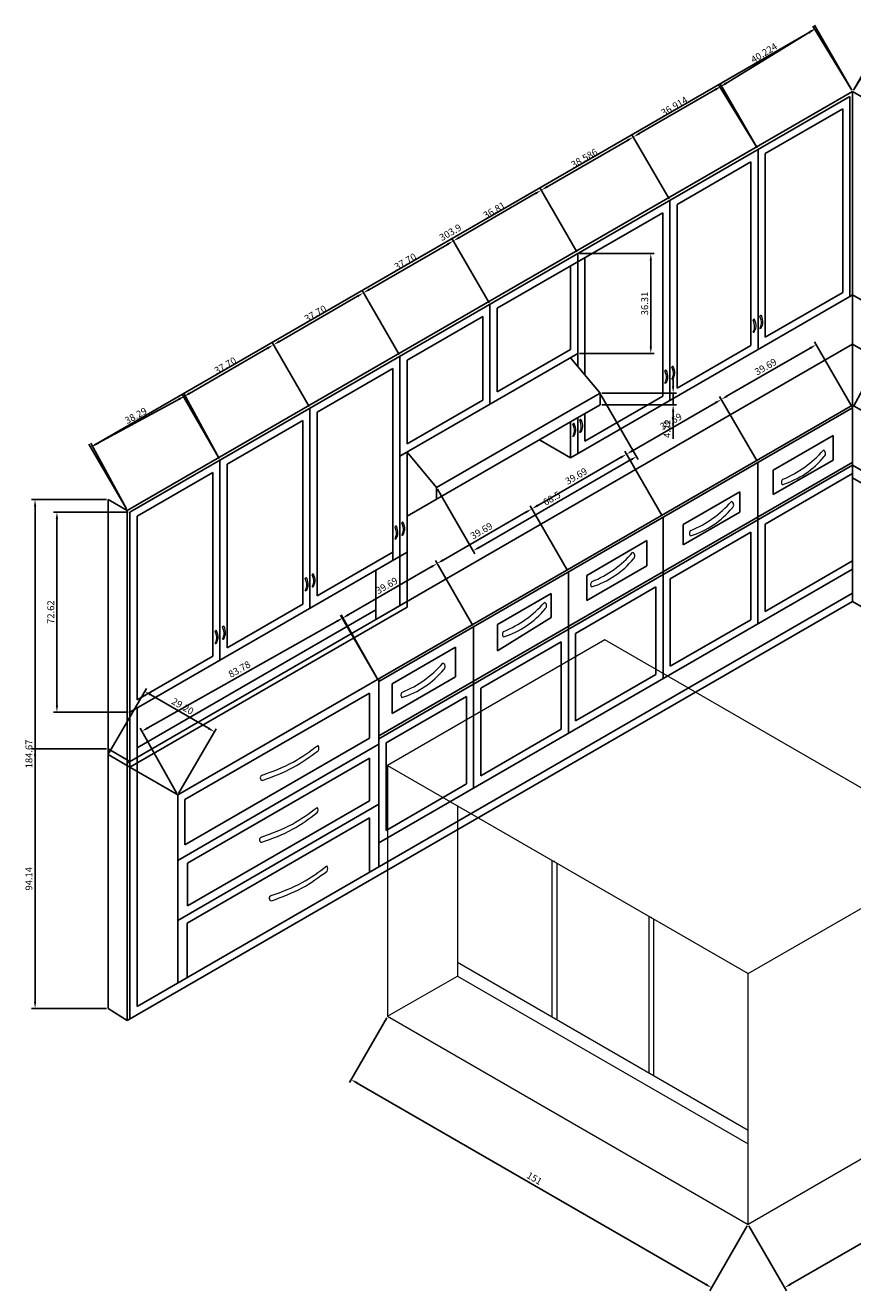
# Model space of a CAD drawing. Units: centimetres. Extents: x 21667 to 22807, y 15845 to 16565.
# Tile 3 of 4: x 22275 to 22575, y 16106 to 16565. Entities that reach past the tile are written whole.
import ezdxf

# ---------------------------------------------------------------- set-up
doc = ezdxf.new("R2010")
doc.units = ezdxf.units.CM
for name, color, linetype, lineweight in [('A-ANNO-DIMS', 2, 'Continuous', 18), ('A-ANNO-NPLT', 8, 'Continuous', 13), ('A-FURN', 8, 'Continuous', 18), ('A-FURN-CASE', 7, 'Continuous', 25), ('A-FURN-HDWR', 8, 'Continuous', 13)]:
    doc.layers.add(name, color=color, linetype=linetype, lineweight=lineweight)
doc.styles.get("Standard").update_dxf_attribs({"font": 'arial.ttf'})
doc.dimstyles.new('ISO-25', dxfattribs={"dimtxt": 2.5, "dimasz": 2.5, "dimexe": 1.25, "dimexo": 0.625, "dimtad": 1, "dimtxsty": 'Standard', "dimcen": 2.5, "dimadec": 0, "dimazin": 0, "dimtfac": 1, "dimtmove": 0, "dimatfit": 3, "dimfxl": 1, "dimarcsym": 0})

# ---------------------------------------------------------------- blocks, each defined once
blk = doc.blocks.new('hanger')
for centre, radius, start, end in [((22344.01, 16340.62), 0.329, 55.972, 165.7251), ((22343.56, 16337.35), 1.11, 276.778, 304.9191)]:
    blk.add_arc(centre, radius, start, end)
for points, knots in [([(22343.69, 16336.25), (22343.94, 16336.83), (22344.57, 16338.28), (22344.02, 16339.79), (22343.69, 16340.7)], [0, 0, 0, 0, 1.834135, 4.5977, 4.5977, 4.5977, 4.5977]), ([(22344.2, 16336.44), (22344.45, 16337.04), (22345.07, 16338.5), (22344.52, 16340.01), (22344.2, 16340.89)], [0, 0, 0, 0, 1.89598, 4.599425, 4.599425, 4.599425, 4.599425])]:
    blk.add_open_spline(points, degree=3, knots=knots)
blk = doc.blocks.new('tabl e3')
for p, q in [((22512.57, 16212.95), (22433.76, 16167.45)), ((22643.34, 16137.45), (22512.57, 16212.95)), ((22433.76, 16167.45), (22564.53, 16091.95)), ((22433.76, 16167.45), (22433.76, 16076.45)), ((22459.07, 16152.84), (22459.07, 16091.06)), ((22564.53, 16091.95), (22643.34, 16137.45)), ((22643.34, 16137.45), (22643.34, 16046.45)), ((22493.36, 16133.04), (22493.36, 16076.26)), ((22495.09, 16132.04), (22495.09, 16075.26)), ((22528.51, 16112.74), (22528.51, 16055.97)), ((22530.25, 16111.74), (22530.25, 16054.97)), ((22459.07, 16096.06), (22564.53, 16035.17)), ((22433.76, 16076.45), (22459.07, 16091.06)), ((22459.07, 16091.06), (22564.53, 16030.17)), ((22564.53, 16000.95), (22564.53, 16091.95)), ((22433.76, 16076.45), (22564.53, 16000.95)), ((22643.34, 16046.45), (22564.53, 16000.95))]:
    blk.add_line(p, q)
for p in [(22494.23, 16132.54), (22529.38, 16112.24)]:
    blk.add_point(p)
blk = doc.blocks.new('PULL-KNOB-D')
for centre, radius, start, end in [((19.64, 11.69), 1.63, 325.6763, 37.1687), ((0.97, 0.96), 0.968, 101.3534, 261.4916)]:
    blk.add_arc(centre, radius, start, end)
for points in [[(0.78, 1.91), (4.6, 3.31), (11.83, 5.95), (18.02, 10.52), (20.94, 12.67)], [(0.82, 0), (4.64, 1.4), (11.87, 4.05), (18.07, 8.61), (20.99, 10.77)]]:
    blk.add_open_spline(points, degree=3, knots=[0, 0, 0, 0, 12.131271, 22.961741, 22.961741, 22.961741, 22.961741])
blk = doc.blocks.new('DRAWER-PULL')
for centre, radius, start, end in [((-9.25, 30.72), 32.2, 287.3997, 320.4809), ((-14.25, 38.11), 39.06, 292.2568, 319.0454), ((14.72, 11.27), 1.35, 309.9814, 67.0584), ((1.29, 0.92), 1.29, 125.3328, 225.1316)]:
    blk.add_arc(centre, radius, start, end)
blk = doc.blocks.new('*D26')
at = {"layer": 'A-ANNO-DIMS', "color": 0, "lineweight": -2, "transparency": 16777216}
for p, q in [((22574.64, 16541.62), (22561.08, 16565.11)), ((22300.7, 16413.33), (22559.54, 16562.77)), ((22311.47, 16389.67), (22297.91, 16413.17))]:
    blk.add_line(p, q, dxfattribs=at)
at = {"layer": 'A-ANNO-DIMS', "color": 0, "transparency": 16777216}
for points in [[(22559.33, 16563.14), (22559.75, 16562.41), (22561.7, 16564.02)], [(22300.49, 16413.69), (22300.9, 16412.97), (22298.53, 16412.08)]]:
    blk.add_solid(points, dxfattribs=at)
at = {"layer": 'Defpoints', "color": 0, "transparency": 16777216}
for p in [(22561.7, 16564.02), (22574.95, 16541.07), (22311.78, 16389.13)]:
    blk.add_point(p, dxfattribs=at)
at = {"layer": 'A-ANNO-DIMS', "color": 0, "transparency": 16777216, "insert": (22429.17, 16489.7), "char_height": 2.5, "attachment_point": 5, "rotation": 30}
blk.add_mtext('303.9', dxfattribs=at)
blk = doc.blocks.new('*D27')
at = {"layer": 'A-ANNO-DIMS', "color": 0, "lineweight": -2, "transparency": 16777216}
for p, q in [((22575.26, 16541.62), (22588.83, 16565.11)), ((22590.37, 16562.77), (22793.02, 16445.77)), ((22782.24, 16422.12), (22795.81, 16445.61))]:
    blk.add_line(p, q, dxfattribs=at)
at = {"layer": 'A-ANNO-DIMS', "color": 0, "transparency": 16777216}
for points in [[(22590.58, 16563.14), (22590.16, 16562.41), (22588.2, 16564.02)], [(22793.23, 16446.14), (22792.81, 16445.41), (22795.18, 16444.52)]]:
    blk.add_solid(points, dxfattribs=at)
at = {"layer": 'Defpoints', "color": 0, "transparency": 16777216}
for p in [(22574.95, 16541.07), (22795.18, 16444.52), (22781.93, 16421.57)]:
    blk.add_point(p, dxfattribs=at)
at = {"layer": 'A-ANNO-DIMS', "color": 0, "transparency": 16777216, "insert": (22692.64, 16505.92), "char_height": 2.5, "attachment_point": 5, "rotation": 330}
blk.add_mtext('239', dxfattribs=at)
blk = doc.blocks.new('*D28')
at = {"layer": 'A-ANNO-DIMS', "color": 0, "lineweight": -2, "transparency": 16777216}
for p, q in [((22304.23, 16393.13), (22277.1, 16393.13)), ((22278.35, 16210.96), (22278.35, 16390.63)), ((22304.23, 16208.46), (22277.1, 16208.46))]:
    blk.add_line(p, q, dxfattribs=at)
at = {"layer": 'A-ANNO-DIMS', "color": 0, "transparency": 16777216}
for points in [[(22277.94, 16390.63), (22278.77, 16390.63), (22278.35, 16393.13)], [(22277.94, 16210.96), (22278.77, 16210.96), (22278.35, 16208.46)]]:
    blk.add_solid(points, dxfattribs=at)
at = {"layer": 'Defpoints', "color": 0, "transparency": 16777216}
for p in [(22278.35, 16393.13), (22304.85, 16393.13), (22304.85, 16208.46)]:
    blk.add_point(p, dxfattribs=at)
at = {"layer": 'A-ANNO-DIMS', "color": 0, "transparency": 16777216, "insert": (22276.45, 16300.8), "char_height": 2.5, "attachment_point": 5, "rotation": 90}
blk.add_mtext('184.67', dxfattribs=at)
blk = doc.blocks.new('*D29')
at = {"layer": 'A-ANNO-DIMS', "color": 0, "lineweight": -2, "transparency": 16777216}
for p, q in [((22304.23, 16302.61), (22277.1, 16302.61)), ((22278.35, 16210.96), (22278.35, 16300.11)), ((22304.23, 16208.46), (22277.1, 16208.46))]:
    blk.add_line(p, q, dxfattribs=at)
at = {"layer": 'A-ANNO-DIMS', "color": 0, "transparency": 16777216}
for points in [[(22277.94, 16300.11), (22278.77, 16300.11), (22278.35, 16302.61)], [(22277.94, 16210.96), (22278.77, 16210.96), (22278.35, 16208.46)]]:
    blk.add_solid(points, dxfattribs=at)
at = {"layer": 'Defpoints', "color": 0, "transparency": 16777216}
for p in [(22278.35, 16302.61), (22304.85, 16302.61), (22304.85, 16208.46)]:
    blk.add_point(p, dxfattribs=at)
at = {"layer": 'A-ANNO-DIMS', "color": 0, "transparency": 16777216, "insert": (22276.45, 16255.53), "char_height": 2.5, "attachment_point": 5, "rotation": 90}
blk.add_mtext('94.14', dxfattribs=at)
blk = doc.blocks.new('*D30')
at = {"layer": 'A-ANNO-DIMS', "color": 0, "lineweight": -2, "transparency": 16777216}
for p, q in [((22312.16, 16388.56), (22285.03, 16388.56)), ((22286.28, 16318.44), (22286.28, 16386.06)), ((22312.16, 16315.94), (22285.03, 16315.94))]:
    blk.add_line(p, q, dxfattribs=at)
at = {"layer": 'A-ANNO-DIMS', "color": 0, "transparency": 16777216}
for points in [[(22285.86, 16386.06), (22286.7, 16386.06), (22286.28, 16388.56)], [(22285.86, 16318.44), (22286.7, 16318.44), (22286.28, 16315.94)]]:
    blk.add_solid(points, dxfattribs=at)
at = {"layer": 'Defpoints', "color": 0, "transparency": 16777216}
for p in [(22286.28, 16388.56), (22312.78, 16388.56), (22312.78, 16315.94)]:
    blk.add_point(p, dxfattribs=at)
at = {"layer": 'A-ANNO-DIMS', "color": 0, "transparency": 16777216, "insert": (22284.38, 16352.25), "char_height": 2.5, "attachment_point": 5, "rotation": 90}
blk.add_mtext('72.62', dxfattribs=at)
blk = doc.blocks.new('*D31')
at = {"layer": 'A-ANNO-DIMS', "color": 0, "lineweight": -2, "transparency": 16777216}
for p, q in [((22483.65, 16431.12), (22497.21, 16407.63)), ((22494.42, 16407.46), (22439.42, 16375.71)), ((22424.32, 16396.87), (22437.88, 16373.38))]:
    blk.add_line(p, q, dxfattribs=at)
at = {"layer": 'A-ANNO-DIMS', "color": 0, "transparency": 16777216}
for points in [[(22494.21, 16407.82), (22494.63, 16407.1), (22496.58, 16408.71)], [(22439.21, 16376.07), (22439.63, 16375.35), (22437.26, 16374.46)]]:
    blk.add_solid(points, dxfattribs=at)
at = {"layer": 'Defpoints', "color": 0, "transparency": 16777216}
for p in [(22483.33, 16431.66), (22424.01, 16397.41), (22437.26, 16374.46)]:
    blk.add_point(p, dxfattribs=at)
at = {"layer": 'A-ANNO-DIMS', "color": 0, "transparency": 16777216, "insert": (22465.97, 16393.23), "char_height": 2.5, "attachment_point": 5, "rotation": 30}
blk.add_mtext('68.5', dxfattribs=at)
blk = doc.blocks.new('*D34')
at = {"layer": 'A-ANNO-DIMS', "color": 0, "lineweight": -2, "transparency": 16777216}
for p, q in [((22405.95, 16205.11), (22392.39, 16181.62)), ((22521.62, 16108.45), (22395.18, 16181.45)), ((22536.72, 16129.61), (22523.16, 16106.12))]:
    blk.add_line(p, q, dxfattribs=at)
at = {"layer": 'A-ANNO-DIMS', "color": 0, "transparency": 16777216}
for points in [[(22395.39, 16181.81), (22394.97, 16181.09), (22393.01, 16182.7)], [(22521.83, 16108.81), (22521.41, 16108.09), (22523.78, 16107.2)]]:
    blk.add_solid(points, dxfattribs=at)
at = {"layer": 'Defpoints', "color": 0, "transparency": 16777216}
for p in [(22406.26, 16205.65), (22393.01, 16182.7), (22537.03, 16130.15)]:
    blk.add_point(p, dxfattribs=at)
at = {"layer": 'A-ANNO-DIMS', "color": 0, "transparency": 16777216, "insert": (22459.35, 16146.59), "char_height": 2.5, "attachment_point": 5, "rotation": 330}
blk.add_mtext('151', dxfattribs=at)
blk = doc.blocks.new('*D35')
at = {"layer": 'A-ANNO-DIMS', "color": 0, "lineweight": -2, "transparency": 16777216}
for p, q in [((22616.15, 16175.11), (22629.72, 16151.62)), ((22626.93, 16151.45), (22552.45, 16108.45)), ((22537.35, 16129.61), (22550.91, 16106.12))]:
    blk.add_line(p, q, dxfattribs=at)
at = {"layer": 'A-ANNO-DIMS', "color": 0, "transparency": 16777216}
for points in [[(22626.72, 16151.81), (22627.14, 16151.09), (22629.09, 16152.7)], [(22552.24, 16108.81), (22552.66, 16108.09), (22550.28, 16107.2)]]:
    blk.add_solid(points, dxfattribs=at)
at = {"layer": 'Defpoints', "color": 0, "transparency": 16777216}
for p in [(22615.84, 16175.65), (22537.03, 16130.15), (22550.28, 16107.2)]:
    blk.add_point(p, dxfattribs=at)
at = {"layer": 'A-ANNO-DIMS', "color": 0, "transparency": 16777216, "insert": (22588.74, 16131.59), "char_height": 2.5, "attachment_point": 5, "rotation": 30}
blk.add_mtext('91', dxfattribs=at)
blk = doc.blocks.new('*D54')
at = {"layer": 'A-ANNO-DIMS', "color": 0, "lineweight": -2, "transparency": 16777216}
for p, q in [((22301.33, 16413.61), (22330.58, 16429.5)), ((22345.13, 16407.95), (22332.18, 16431.79)), ((22311.48, 16389.68), (22298.54, 16413.52))]:
    blk.add_line(p, q, dxfattribs=at)
at = {"layer": 'A-ANNO-DIMS', "color": 0, "transparency": 16777216}
for points in [[(22330.38, 16429.86), (22330.78, 16429.13), (22332.78, 16430.69)], [(22301.13, 16413.98), (22301.53, 16413.25), (22299.13, 16412.42)]]:
    blk.add_solid(points, dxfattribs=at)
at = {"layer": 'Defpoints', "color": 0, "transparency": 16777216}
for p in [(22332.78, 16430.69), (22345.43, 16407.4), (22311.78, 16389.13)]:
    blk.add_point(p, dxfattribs=at)
at = {"layer": 'A-ANNO-DIMS', "color": 0, "transparency": 16777216, "insert": (22315.05, 16423.23), "char_height": 2.5, "attachment_point": 5, "rotation": 28.5034}
blk.add_mtext('38.29', dxfattribs=at)
blk = doc.blocks.new('*D55')
at = {"layer": 'A-ANNO-DIMS', "color": 0, "lineweight": -2, "transparency": 16777216}
for p, q in [((22377.76, 16426.79), (22364.2, 16450.28)), ((22334.34, 16431.6), (22362.66, 16447.95)), ((22345.11, 16407.95), (22331.55, 16431.44))]:
    blk.add_line(p, q, dxfattribs=at)
at = {"layer": 'A-ANNO-DIMS', "color": 0, "transparency": 16777216}
for points in [[(22362.45, 16448.31), (22362.87, 16447.59), (22364.82, 16449.2)], [(22334.13, 16431.96), (22334.55, 16431.24), (22332.18, 16430.35)]]:
    blk.add_solid(points, dxfattribs=at)
at = {"layer": 'Defpoints', "color": 0, "transparency": 16777216}
for p in [(22364.82, 16449.2), (22378.07, 16426.25), (22345.43, 16407.4)]:
    blk.add_point(p, dxfattribs=at)
at = {"layer": 'A-ANNO-DIMS', "color": 0, "transparency": 16777216, "insert": (22347.55, 16441.43), "char_height": 2.5, "attachment_point": 5, "rotation": 30}
blk.add_mtext('37.70', dxfattribs=at)
blk = doc.blocks.new('*D56')
at = {"layer": 'A-ANNO-DIMS', "color": 0, "lineweight": -2, "transparency": 16777216}
for p, q in [((22410.41, 16445.64), (22396.84, 16469.13)), ((22366.99, 16450.45), (22395.3, 16466.8)), ((22377.76, 16426.79), (22364.2, 16450.28))]:
    blk.add_line(p, q, dxfattribs=at)
at = {"layer": 'A-ANNO-DIMS', "color": 0, "transparency": 16777216}
for points in [[(22395.1, 16467.16), (22395.51, 16466.44), (22397.47, 16468.05)], [(22366.78, 16450.81), (22367.2, 16450.09), (22364.82, 16449.2)]]:
    blk.add_solid(points, dxfattribs=at)
at = {"layer": 'Defpoints', "color": 0, "transparency": 16777216}
for p in [(22397.47, 16468.05), (22410.72, 16445.1), (22378.07, 16426.25)]:
    blk.add_point(p, dxfattribs=at)
at = {"layer": 'A-ANNO-DIMS', "color": 0, "transparency": 16777216, "insert": (22380.2, 16460.27), "char_height": 2.5, "attachment_point": 5, "rotation": 30}
blk.add_mtext('37.70', dxfattribs=at)
blk = doc.blocks.new('*D57')
at = {"layer": 'A-ANNO-DIMS', "color": 0, "lineweight": -2, "transparency": 16777216}
for p, q in [((22443.05, 16464.49), (22429.49, 16487.98)), ((22399.63, 16469.3), (22427.95, 16485.65)), ((22410.41, 16445.64), (22396.84, 16469.13))]:
    blk.add_line(p, q, dxfattribs=at)
at = {"layer": 'A-ANNO-DIMS', "color": 0, "transparency": 16777216}
for points in [[(22427.74, 16486.01), (22428.16, 16485.29), (22430.12, 16486.9)], [(22399.43, 16469.66), (22399.84, 16468.94), (22397.47, 16468.05)]]:
    blk.add_solid(points, dxfattribs=at)
at = {"layer": 'Defpoints', "color": 0, "transparency": 16777216}
for p in [(22430.12, 16486.9), (22443.37, 16463.95), (22410.72, 16445.1)]:
    blk.add_point(p, dxfattribs=at)
at = {"layer": 'A-ANNO-DIMS', "color": 0, "transparency": 16777216, "insert": (22412.84, 16479.12), "char_height": 2.5, "attachment_point": 5, "rotation": 30}
blk.add_mtext('37.70', dxfattribs=at)
blk = doc.blocks.new('*D58')
at = {"layer": 'A-ANNO-DIMS', "color": 0, "lineweight": -2, "transparency": 16777216}
for p, q in [((22474.93, 16482.89), (22461.37, 16506.39)), ((22432.28, 16488.15), (22459.83, 16504.05)), ((22443.05, 16464.49), (22429.49, 16487.98))]:
    blk.add_line(p, q, dxfattribs=at)
at = {"layer": 'A-ANNO-DIMS', "color": 0, "transparency": 16777216}
for points in [[(22459.62, 16504.41), (22460.04, 16503.69), (22461.99, 16505.3)], [(22432.07, 16488.51), (22432.49, 16487.79), (22430.12, 16486.9)]]:
    blk.add_solid(points, dxfattribs=at)
at = {"layer": 'Defpoints', "color": 0, "transparency": 16777216}
for p in [(22461.99, 16505.3), (22475.24, 16482.35), (22443.37, 16463.95)]:
    blk.add_point(p, dxfattribs=at)
at = {"layer": 'A-ANNO-DIMS', "color": 0, "transparency": 16777216, "insert": (22445.1, 16497.75), "char_height": 2.5, "attachment_point": 5, "rotation": 30}
blk.add_mtext('36.81', dxfattribs=at)
blk = doc.blocks.new('*D59')
at = {"layer": 'A-ANNO-DIMS', "color": 0, "lineweight": -2, "transparency": 16777216}
for p, q in [((22508.35, 16502.19), (22494.78, 16525.68)), ((22464.16, 16506.55), (22493.24, 16523.35)), ((22474.93, 16482.89), (22461.37, 16506.39))]:
    blk.add_line(p, q, dxfattribs=at)
at = {"layer": 'A-ANNO-DIMS', "color": 0, "transparency": 16777216}
for points in [[(22493.04, 16523.71), (22493.45, 16522.98), (22495.41, 16524.6)], [(22463.95, 16506.91), (22464.37, 16506.19), (22461.99, 16505.3)]]:
    blk.add_solid(points, dxfattribs=at)
at = {"layer": 'Defpoints', "color": 0, "transparency": 16777216}
for p in [(22495.41, 16524.6), (22508.66, 16501.65), (22475.24, 16482.35)]:
    blk.add_point(p, dxfattribs=at)
at = {"layer": 'A-ANNO-DIMS', "color": 0, "transparency": 16777216, "insert": (22477.75, 16516.6), "char_height": 2.5, "attachment_point": 5, "rotation": 30}
blk.add_mtext('38.586', dxfattribs=at)
blk = doc.blocks.new('*D60')
at = {"layer": 'A-ANNO-DIMS', "color": 0, "lineweight": -2, "transparency": 16777216}
for p, q in [((22540.32, 16520.64), (22526.75, 16544.14)), ((22497.57, 16525.85), (22525.21, 16541.8)), ((22508.35, 16502.19), (22494.78, 16525.68))]:
    blk.add_line(p, q, dxfattribs=at)
at = {"layer": 'A-ANNO-DIMS', "color": 0, "transparency": 16777216}
for points in [[(22525, 16542.16), (22525.42, 16541.44), (22527.38, 16543.05)], [(22497.37, 16526.21), (22497.78, 16525.48), (22495.41, 16524.6)]]:
    blk.add_solid(points, dxfattribs=at)
at = {"layer": 'Defpoints', "color": 0, "transparency": 16777216}
for p in [(22527.38, 16543.05), (22540.63, 16520.1), (22508.66, 16501.65)]:
    blk.add_point(p, dxfattribs=at)
at = {"layer": 'A-ANNO-DIMS', "color": 0, "transparency": 16777216, "insert": (22510.44, 16535.47), "char_height": 2.5, "attachment_point": 5, "rotation": 30}
blk.add_mtext('36.914', dxfattribs=at)
blk = doc.blocks.new('*D61')
at = {"layer": 'A-ANNO-DIMS', "color": 0, "lineweight": -2, "transparency": 16777216}
for p, q in [((22528.94, 16544.02), (22559, 16562.38)), ((22574.63, 16541.61), (22560.48, 16564.75)), ((22540.3, 16520.64), (22526.16, 16543.78))]:
    blk.add_line(p, q, dxfattribs=at)
at = {"layer": 'A-ANNO-DIMS', "color": 0, "transparency": 16777216}
for points in [[(22558.78, 16562.74), (22559.22, 16562.03), (22561.14, 16563.69)], [(22528.73, 16544.38), (22529.16, 16543.66), (22526.81, 16542.72)]]:
    blk.add_solid(points, dxfattribs=at)
at = {"layer": 'Defpoints', "color": 0, "transparency": 16777216}
for p in [(22561.14, 16563.69), (22574.95, 16541.07), (22540.63, 16520.1)]:
    blk.add_point(p, dxfattribs=at)
at = {"layer": 'A-ANNO-DIMS', "color": 0, "transparency": 16777216, "insert": (22542.98, 16554.82), "char_height": 2.5, "attachment_point": 5, "rotation": 31.4246}
blk.add_mtext('40.224', dxfattribs=at)
blk = doc.blocks.new('*D62')
at = {"layer": 'A-ANNO-DIMS', "color": 0, "lineweight": -2, "transparency": 16777216}
for p, q in [((22575.28, 16541.61), (22589.49, 16564.71)), ((22590.96, 16562.34), (22613.38, 16548.56)), ((22601.95, 16525.21), (22616.16, 16548.31))]:
    blk.add_line(p, q, dxfattribs=at)
at = {"layer": 'A-ANNO-DIMS', "color": 0, "transparency": 16777216}
for points in [[(22591.18, 16562.69), (22590.74, 16561.99), (22588.83, 16563.65)], [(22613.59, 16548.91), (22613.16, 16548.2), (22615.51, 16547.25)]]:
    blk.add_solid(points, dxfattribs=at)
at = {"layer": 'Defpoints', "color": 0, "transparency": 16777216}
for p in [(22615.51, 16547.25), (22574.95, 16541.07), (22601.63, 16524.67)]:
    blk.add_point(p, dxfattribs=at)
at = {"layer": 'A-ANNO-DIMS', "color": 0, "transparency": 16777216, "insert": (22603.16, 16557.07), "char_height": 2.5, "attachment_point": 5, "rotation": 328.4151}
blk.add_mtext('31.31', dxfattribs=at)
blk = doc.blocks.new('*D69')
at = {"layer": 'A-ANNO-DIMS', "color": 0, "lineweight": -2, "transparency": 16777216}
for p, q in [((22402.78, 16327.62), (22389.46, 16351.25)), ((22319.27, 16310.25), (22387.9, 16348.93)), ((22329.79, 16286.48), (22316.48, 16310.11))]:
    blk.add_line(p, q, dxfattribs=at)
at = {"layer": 'A-ANNO-DIMS', "color": 0, "transparency": 16777216}
for points in [[(22387.69, 16349.3), (22388.1, 16348.57), (22390.08, 16350.16)], [(22319.06, 16310.61), (22319.47, 16309.89), (22317.09, 16309.02)]]:
    blk.add_solid(points, dxfattribs=at)
at = {"layer": 'Defpoints', "color": 0, "transparency": 16777216}
for p in [(22390.08, 16350.16), (22403.09, 16327.08), (22330.1, 16285.94)]:
    blk.add_point(p, dxfattribs=at)
at = {"layer": 'A-ANNO-DIMS', "color": 0, "transparency": 16777216, "insert": (22352.65, 16331.25), "char_height": 2.5, "attachment_point": 5, "rotation": 29.4078}
blk.add_mtext('83.78', dxfattribs=at)
blk = doc.blocks.new('*D70')
at = {"layer": 'A-ANNO-DIMS', "color": 0, "lineweight": -2, "transparency": 16777216}
for p, q in [((22392, 16351.28), (22422.05, 16368.62)), ((22437.15, 16347.46), (22423.59, 16370.95)), ((22402.78, 16327.62), (22389.21, 16351.11))]:
    blk.add_line(p, q, dxfattribs=at)
at = {"layer": 'A-ANNO-DIMS', "color": 0, "transparency": 16777216}
for points in [[(22421.84, 16368.98), (22422.25, 16368.26), (22424.21, 16369.87)], [(22391.8, 16351.64), (22392.21, 16350.92), (22389.84, 16350.03)]]:
    blk.add_solid(points, dxfattribs=at)
at = {"layer": 'Defpoints', "color": 0, "transparency": 16777216}
for p in [(22424.21, 16369.87), (22437.46, 16346.92), (22403.09, 16327.08)]:
    blk.add_point(p, dxfattribs=at)
at = {"layer": 'A-ANNO-DIMS', "color": 0, "transparency": 16777216, "insert": (22406.07, 16361.6), "char_height": 2.5, "attachment_point": 5, "rotation": 30}
blk.add_mtext('39.69', dxfattribs=at)
blk = doc.blocks.new('*D71')
at = {"layer": 'A-ANNO-DIMS', "color": 0, "lineweight": -2, "transparency": 16777216}
for p, q in [((22471.52, 16367.31), (22457.96, 16390.8)), ((22426.38, 16371.12), (22456.42, 16388.47)), ((22437.15, 16347.46), (22423.59, 16370.95))]:
    blk.add_line(p, q, dxfattribs=at)
at = {"layer": 'A-ANNO-DIMS', "color": 0, "transparency": 16777216}
for points in [[(22456.21, 16388.83), (22456.63, 16388.11), (22458.58, 16389.72)], [(22426.17, 16371.48), (22426.58, 16370.76), (22424.21, 16369.87)]]:
    blk.add_solid(points, dxfattribs=at)
at = {"layer": 'Defpoints', "color": 0, "transparency": 16777216}
for p in [(22458.58, 16389.72), (22471.83, 16366.77), (22437.46, 16346.92)]:
    blk.add_point(p, dxfattribs=at)
at = {"layer": 'A-ANNO-DIMS', "color": 0, "transparency": 16777216, "insert": (22440.45, 16381.44), "char_height": 2.5, "attachment_point": 5, "rotation": 30}
blk.add_mtext('39.69', dxfattribs=at)
blk = doc.blocks.new('*D72')
at = {"layer": 'A-ANNO-DIMS', "color": 0, "lineweight": -2, "transparency": 16777216}
for p, q in [((22505.89, 16387.15), (22492.33, 16410.64)), ((22460.75, 16390.97), (22490.79, 16408.31)), ((22471.52, 16367.31), (22457.96, 16390.8))]:
    blk.add_line(p, q, dxfattribs=at)
at = {"layer": 'A-ANNO-DIMS', "color": 0, "transparency": 16777216}
for points in [[(22490.58, 16408.67), (22491, 16407.95), (22492.96, 16409.56)], [(22460.54, 16391.33), (22460.96, 16390.61), (22458.58, 16389.72)]]:
    blk.add_solid(points, dxfattribs=at)
at = {"layer": 'Defpoints', "color": 0, "transparency": 16777216}
for p in [(22492.96, 16409.56), (22506.21, 16386.61), (22471.83, 16366.77)]:
    blk.add_point(p, dxfattribs=at)
at = {"layer": 'A-ANNO-DIMS', "color": 0, "transparency": 16777216, "insert": (22474.82, 16401.29), "char_height": 2.5, "attachment_point": 5, "rotation": 30}
blk.add_mtext('39.69', dxfattribs=at)
blk = doc.blocks.new('*D73')
at = {"layer": 'A-ANNO-DIMS', "color": 0, "lineweight": -2, "transparency": 16777216}
for p, q in [((22495.12, 16410.81), (22525.16, 16428.16)), ((22540.27, 16407), (22526.7, 16430.49)), ((22505.89, 16387.15), (22492.33, 16410.64))]:
    blk.add_line(p, q, dxfattribs=at)
at = {"layer": 'A-ANNO-DIMS', "color": 0, "transparency": 16777216}
for points in [[(22524.96, 16428.52), (22525.37, 16427.8), (22527.33, 16429.41)], [(22494.91, 16411.17), (22495.33, 16410.45), (22492.96, 16409.56)]]:
    blk.add_solid(points, dxfattribs=at)
at = {"layer": 'Defpoints', "color": 0, "transparency": 16777216}
for p in [(22527.33, 16429.41), (22540.58, 16406.46), (22506.21, 16386.61)]:
    blk.add_point(p, dxfattribs=at)
at = {"layer": 'A-ANNO-DIMS', "color": 0, "transparency": 16777216, "insert": (22509.19, 16421.13), "char_height": 2.5, "attachment_point": 5, "rotation": 30}
blk.add_mtext('39.69', dxfattribs=at)
blk = doc.blocks.new('*D74')
at = {"layer": 'A-ANNO-DIMS', "color": 0, "lineweight": -2, "transparency": 16777216}
for p, q in [((22574.64, 16426.84), (22561.08, 16450.33)), ((22529.49, 16430.66), (22559.54, 16448)), ((22540.27, 16407), (22526.7, 16430.49))]:
    blk.add_line(p, q, dxfattribs=at)
at = {"layer": 'A-ANNO-DIMS', "color": 0, "transparency": 16777216}
for points in [[(22559.33, 16448.36), (22559.75, 16447.64), (22561.7, 16449.25)], [(22529.29, 16431.02), (22529.7, 16430.3), (22527.33, 16429.41)]]:
    blk.add_solid(points, dxfattribs=at)
at = {"layer": 'Defpoints', "color": 0, "transparency": 16777216}
for p in [(22561.7, 16449.25), (22574.95, 16426.3), (22540.58, 16406.46)]:
    blk.add_point(p, dxfattribs=at)
at = {"layer": 'A-ANNO-DIMS', "color": 0, "transparency": 16777216, "insert": (22543.56, 16440.98), "char_height": 2.5, "attachment_point": 5, "rotation": 30}
blk.add_mtext('39.69', dxfattribs=at)
blk = doc.blocks.new('*D75')
at = {"layer": 'A-ANNO-DIMS', "color": 0, "lineweight": -2, "transparency": 16777216}
for p, q in [((22575.25, 16426.85), (22588.1, 16450.74)), ((22589.71, 16448.45), (22610.71, 16437.16)), ((22600.65, 16413.19), (22613.5, 16437.07))]:
    blk.add_line(p, q, dxfattribs=at)
at = {"layer": 'A-ANNO-DIMS', "color": 0, "transparency": 16777216}
for points in [[(22589.91, 16448.82), (22589.51, 16448.09), (22587.51, 16449.64)], [(22610.91, 16437.52), (22610.51, 16436.79), (22612.91, 16435.97)]]:
    blk.add_solid(points, dxfattribs=at)
at = {"layer": 'Defpoints', "color": 0, "transparency": 16777216}
for p in [(22612.91, 16435.97), (22574.95, 16426.3), (22600.36, 16412.64)]:
    blk.add_point(p, dxfattribs=at)
at = {"layer": 'A-ANNO-DIMS', "color": 0, "transparency": 16777216, "insert": (22601.11, 16444.48), "char_height": 2.5, "attachment_point": 5, "rotation": 331.7204}
blk.add_mtext('28.846', dxfattribs=at)
blk = doc.blocks.new('*D79')
at = {"layer": 'A-ANNO-DIMS', "color": 0, "lineweight": -2, "transparency": 16777216}
for p, q in [((22305.17, 16301.15), (22318.79, 16324.6)), ((22320.33, 16322.26), (22341.25, 16310.11)), ((22330.41, 16286.48), (22344.04, 16309.93))]:
    blk.add_line(p, q, dxfattribs=at)
at = {"layer": 'A-ANNO-DIMS', "color": 0, "transparency": 16777216}
for points in [[(22320.54, 16322.62), (22320.12, 16321.9), (22318.16, 16323.52)], [(22341.46, 16310.47), (22341.04, 16309.75), (22343.41, 16308.85)]]:
    blk.add_solid(points, dxfattribs=at)
at = {"layer": 'Defpoints', "color": 0, "transparency": 16777216}
for p in [(22343.41, 16308.85), (22304.85, 16300.61), (22330.1, 16285.94)]:
    blk.add_point(p, dxfattribs=at)
at = {"layer": 'A-ANNO-DIMS', "color": 0, "transparency": 16777216, "insert": (22331.74, 16317.83), "char_height": 2.5, "attachment_point": 5, "rotation": 329.8453}
blk.add_mtext('29.20', dxfattribs=at)
blk = doc.blocks.new('*D80')
at = {"layer": 'A-ANNO-DIMS', "color": 0, "lineweight": -2, "transparency": 16777216}
for p, q in [((22509.83, 16434.16), (22509.83, 16436.66)), ((22483.96, 16431.66), (22511.08, 16431.66)), ((22483.96, 16427.45), (22511.08, 16427.45)), ((22509.83, 16431.66), (22509.83, 16427.45)), ((22509.83, 16424.95), (22509.83, 16415.09))]:
    blk.add_line(p, q, dxfattribs=at)
at = {"layer": 'A-ANNO-DIMS', "color": 0, "transparency": 16777216}
for points in [[(22509.42, 16434.16), (22510.25, 16434.16), (22509.83, 16431.66)], [(22509.42, 16424.95), (22510.25, 16424.95), (22509.83, 16427.45)]]:
    blk.add_solid(points, dxfattribs=at)
at = {"layer": 'Defpoints', "color": 0, "transparency": 16777216}
for p in [(22483.33, 16431.66), (22483.33, 16427.45), (22509.83, 16427.45)]:
    blk.add_point(p, dxfattribs=at)
at = {"layer": 'A-ANNO-DIMS', "color": 0, "transparency": 16777216, "insert": (22507.95, 16418.77), "char_height": 2.5, "attachment_point": 5, "rotation": 90}
blk.add_mtext('4.21', dxfattribs=at)
blk = doc.blocks.new('*D81')
at = {"layer": 'A-ANNO-DIMS', "color": 0, "lineweight": -2, "transparency": 16777216}
for p, q in [((22475.87, 16482.35), (22502.99, 16482.35)), ((22501.74, 16479.85), (22501.74, 16448.54)), ((22475.87, 16446.04), (22502.99, 16446.04))]:
    blk.add_line(p, q, dxfattribs=at)
at = {"layer": 'A-ANNO-DIMS', "color": 0, "transparency": 16777216}
for points in [[(22501.33, 16479.85), (22502.16, 16479.85), (22501.74, 16482.35)], [(22501.33, 16448.54), (22502.16, 16448.54), (22501.74, 16446.04)]]:
    blk.add_solid(points, dxfattribs=at)
at = {"layer": 'Defpoints', "color": 0, "transparency": 16777216}
for p in [(22475.24, 16482.35), (22475.24, 16446.04), (22501.74, 16446.04)]:
    blk.add_point(p, dxfattribs=at)
at = {"layer": 'A-ANNO-DIMS', "color": 0, "transparency": 16777216, "insert": (22499.84, 16464.2), "char_height": 2.5, "attachment_point": 5, "rotation": 90}
blk.add_mtext('36.31', dxfattribs=at)

msp = doc.modelspace()

# ---------------------------------------------------------------- linework, layer by layer
at = {"layer": 'A-ANNO-NPLT'}
for p in [(22540.5793, 16406.4567), (22506.2067, 16386.6116), (22471.8341, 16366.7666), (22437.4615, 16346.9215), (22403.0888, 16304.3343), (22403.0888, 16280.592)]:
    msp.add_point(p, dxfattribs=at)
at = {"layer": 'A-FURN-CASE'}
for p, q in [((22311.7804, 16389.1328), (22574.9519, 16541.075)), ((22312.7804, 16388.5554), (22573.9519, 16539.3429)), ((22573.9519, 16466.7244), (22573.9519, 16539.3429)), ((22574.9519, 16467.3017), (22574.9519, 16541.075)), ((22574.9519, 16541.075), (22705.7218, 16465.575)), ((22543.2257, 16518.6031), (22571.3539, 16534.8429)), ((22571.3539, 16468.2244), (22571.3539, 16534.8429)), ((22540.6276, 16520.1031), (22540.6276, 16447.4846)), ((22511.2571, 16500.146), (22538.0295, 16515.6031)), ((22538.0295, 16515.6031), (22538.0295, 16448.9846)), ((22543.2257, 16518.6031), (22543.2257, 16451.9846)), ((22508.6591, 16501.646), (22508.6591, 16429.0275)), ((22445.9642, 16462.4492), (22506.061, 16497.146)), ((22506.061, 16497.146), (22506.061, 16430.5275)), ((22511.2571, 16500.146), (22511.2571, 16433.5275)), ((22472.6446, 16477.8531), (22472.6446, 16447.5438)), ((22475.2427, 16482.3531), (22475.2427, 16441.4125)), ((22477.8408, 16480.8531), (22477.8408, 16438.2812)), ((22472.6446, 16408.2346), (22573.9519, 16466.7244)), ((22543.2257, 16451.9846), (22571.3539, 16468.2244)), ((22573.9519, 16466.7244), (22574.9519, 16467.3017)), ((22574.9519, 16467.3017), (22705.7218, 16391.8017)), ((22574.9519, 16467.3017), (22574.9519, 16356.075)), ((22413.3178, 16443.6007), (22440.7681, 16459.4492)), ((22440.7681, 16459.4492), (22440.7681, 16429.1399)), ((22443.3662, 16463.9492), (22443.3662, 16427.6399)), ((22445.9642, 16462.4492), (22445.9642, 16432.1399)), ((22311.7804, 16297.4506), (22574.9519, 16449.3927)), ((22410.7197, 16408.7915), (22475.2427, 16446.0438)), ((22445.9642, 16432.1399), (22472.6446, 16447.5438)), ((22511.2571, 16433.5275), (22538.0295, 16448.9846)), ((22574.9519, 16449.3927), (22705.7218, 16373.8927)), ((22410.7197, 16445.1007), (22410.7197, 16354.5732)), ((22413.3178, 16443.6007), (22413.3178, 16413.2915)), ((22472.6446, 16444.5438), (22483.3337, 16431.6608)), ((22380.6714, 16424.7523), (22408.1217, 16440.6007)), ((22408.1217, 16440.6007), (22408.1217, 16370.9822)), ((22413.3178, 16413.2915), (22440.7681, 16429.1399)), ((22472.6446, 16425.4895), (22483.3337, 16431.6608)), ((22472.6446, 16421.276), (22483.3337, 16427.4473)), ((22477.8408, 16414.2346), (22506.061, 16430.5275)), ((22483.3337, 16431.6608), (22483.3337, 16427.4473)), ((22330.1009, 16285.9369), (22574.9519, 16427.3017)), ((22378.0733, 16426.2523), (22378.0733, 16353.6338)), ((22380.6714, 16424.7523), (22380.6714, 16358.1338)), ((22403.0888, 16327.0765), (22574.9519, 16426.3017)), ((22424.0068, 16397.4085), (22472.6446, 16425.4895)), ((22475.2427, 16422.776), (22475.2427, 16409.7346)), ((22477.8408, 16424.276), (22477.8408, 16414.2346)), ((22574.9519, 16427.3017), (22705.7218, 16351.8017)), ((22574.9519, 16427.3017), (22651.1622, 16383.3017)), ((22348.0249, 16405.9039), (22375.4752, 16421.7523)), ((22375.4752, 16421.7523), (22375.4752, 16355.1338)), ((22413.3178, 16387.0237), (22472.6446, 16421.276)), ((22472.6446, 16421.276), (22472.6446, 16408.2346)), ((22472.6446, 16408.2346), (22461.3504, 16414.7553)), ((22567.8403, 16416.2928), (22546.1525, 16403.7714)), ((22567.8403, 16407.4075), (22567.8403, 16416.2928)), ((22413.3178, 16410.2915), (22413.3178, 16354.0732)), ((22413.3178, 16410.2915), (22424.0068, 16397.4085)), ((22345.4268, 16407.4039), (22345.4268, 16334.7853)), ((22348.0249, 16405.9039), (22348.0249, 16339.2853)), ((22403.0888, 16307.3461), (22575.0103, 16406.605)), ((22403.0888, 16306.3343), (22574.9519, 16405.5595)), ((22540.5793, 16406.4567), (22540.5793, 16347.9583)), ((22546.1525, 16394.886), (22567.8403, 16407.4075)), ((22574.9519, 16405.5595), (22651.1622, 16361.5595)), ((22315.3785, 16387.0554), (22342.8288, 16402.9039)), ((22342.8288, 16402.9039), (22342.8288, 16336.2853)), ((22543.1774, 16384.2144), (22574.9519, 16402.5595)), ((22546.1525, 16403.7714), (22546.1525, 16394.886)), ((22574.9519, 16400.9426), (22598.6233, 16387.2759)), ((22424.0068, 16397.4085), (22424.0068, 16393.195)), ((22513.4956, 16384.0636), (22534.0322, 16395.9204)), ((22534.0322, 16395.9204), (22534.0322, 16388.546)), ((22311.7804, 16389.1328), (22304.8522, 16393.1328)), ((22304.8522, 16393.1328), (22304.8522, 16208.4638)), ((22311.7804, 16204.1328), (22311.7804, 16389.1328)), ((22312.7804, 16204.7102), (22312.7804, 16388.5554)), ((22315.3785, 16320.4369), (22315.3785, 16387.0554)), ((22506.2067, 16386.6116), (22506.2067, 16328.1133)), ((22534.0322, 16388.546), (22513.4956, 16376.6891)), ((22513.4956, 16376.6891), (22513.4956, 16384.0636)), ((22543.1774, 16384.2144), (22543.1774, 16352.4583)), ((22478.4723, 16365.582), (22500.3282, 16378.2006)), ((22500.3282, 16378.2006), (22500.3282, 16369.0284)), ((22508.8048, 16364.3694), (22537.9812, 16381.2144)), ((22537.9812, 16381.2144), (22537.9812, 16349.4583)), ((22312.7804, 16315.9369), (22413.3178, 16373.9822)), ((22380.6714, 16358.1338), (22408.1217, 16373.9822)), ((22403.0888, 16268.5782), (22574.9519, 16367.8034)), ((22500.3282, 16369.0284), (22478.4723, 16356.4098)), ((22543.1774, 16352.4583), (22574.9519, 16370.8034)), ((22401.9587, 16367.424), (22401.9587, 16349.515)), ((22471.8341, 16366.7666), (22471.8341, 16308.2683)), ((22478.4723, 16356.4098), (22478.4723, 16365.582)), ((22508.8048, 16364.3694), (22508.8048, 16332.6133)), ((22574.9519, 16359.075), (22315.3785, 16209.2102)), ((22446.0905, 16347.7623), (22465.5913, 16359.0211)), ((22465.5913, 16359.0211), (22465.5913, 16350.3503)), ((22474.4322, 16344.5243), (22503.6086, 16361.3694)), ((22503.6086, 16361.3694), (22503.6086, 16329.6133)), ((22574.9519, 16356.075), (22311.7804, 16204.1328)), ((22312.7804, 16296.0279), (22413.3178, 16354.0732)), ((22348.0249, 16339.2853), (22375.4752, 16355.1338)), ((22705.7218, 16280.575), (22574.9519, 16356.075)), ((22315.3785, 16303.0746), (22401.9587, 16353.0617)), ((22465.5913, 16350.3503), (22446.0905, 16338.2227)), ((22508.8048, 16332.6133), (22537.9812, 16349.4583)), ((22437.4615, 16346.9215), (22437.4615, 16288.4232)), ((22446.0905, 16338.2227), (22446.0905, 16347.7623)), ((22440.0595, 16324.6793), (22469.236, 16341.5243)), ((22469.236, 16341.5243), (22469.236, 16309.7683)), ((22474.4322, 16344.5243), (22474.4322, 16312.7683)), ((22315.3785, 16320.4369), (22342.8288, 16336.2853)), ((22407.8773, 16326.2374), (22430.9262, 16339.5447)), ((22430.9262, 16339.5447), (22430.9262, 16328.728)), ((22403.0888, 16328.0765), (22403.0888, 16259.8498)), ((22430.9262, 16328.728), (22407.8773, 16315.4207)), ((22474.4322, 16312.7683), (22503.6086, 16329.6133)), ((22332.699, 16284.2334), (22399.6579, 16322.8921)), ((22399.6579, 16322.8921), (22399.6579, 16306.4905)), ((22407.8773, 16315.4207), (22407.8773, 16326.2374)), ((22440.0595, 16324.6793), (22440.0595, 16292.9232)), ((22315.3785, 16209.2102), (22315.3785, 16317.4369)), ((22405.6869, 16304.8343), (22434.8634, 16321.6793)), ((22434.8634, 16321.6793), (22434.8634, 16289.9232)), ((22440.0595, 16292.9232), (22469.236, 16309.7683)), ((22403.0888, 16304.3343), (22330.1009, 16262.1947)), ((22399.6579, 16306.4905), (22332.699, 16267.8317)), ((22405.6869, 16304.8343), (22405.6869, 16273.0782)), ((22312.7804, 16298.0279), (22304.8522, 16302.6053)), ((22312.7804, 16296.0279), (22304.8522, 16300.6053)), ((22304.8522, 16300.6053), (22304.8522, 16208.4638)), ((22399.6247, 16299.3343), (22333.6202, 16261.2265)), ((22399.6247, 16299.3343), (22399.6247, 16283.852)), ((22312.7804, 16296.0279), (22330.1009, 16286.0279)), ((22405.6869, 16273.0782), (22434.8634, 16289.9232)), ((22330.1009, 16286.0279), (22330.1009, 16217.7102)), ((22403.0888, 16282.592), (22330.1009, 16240.4524)), ((22332.699, 16284.2334), (22332.699, 16267.8317)), ((22399.6247, 16283.852), (22333.6202, 16245.7443)), ((22399.6247, 16277.592), (22333.565, 16239.4524)), ((22399.6247, 16277.592), (22399.6247, 16257.8498)), ((22333.6202, 16261.2265), (22333.6202, 16245.7443)), ((22333.565, 16239.4524), (22333.565, 16219.7102)), ((22304.8522, 16208.4638), (22311.7804, 16204.1328))]:
    msp.add_line(p, q, dxfattribs=at)

# ---------------------------------------------------------------- block references
at = {"layer": 'A-FURN'}
msp.add_blockref('tabl e3', (-27.5005, 129.1994), dxfattribs=at)
at = {"layer": 'A-FURN-HDWR'}
for name, p in [('hanger', (197.6577, 118.9099)), ('hanger', (195.1513, 117.5098)), ('hanger', (165.6892, 100.4529)), ('hanger', (163.1828, 99.0528)), ('hanger', (129.7664, 79.7598)), ('hanger', (132.2728, 81.1599)), ('DRAWER-PULL', (22549.0903, 16398.4901)), ('DRAWER-PULL', (22515.7373, 16379.9084)), ('hanger', (65.2434, 42.5075)), ('hanger', (67.7498, 43.9076)), ('DRAWER-PULL', (22479.8804, 16361.3774)), ('hanger', (32.7104, 23.7246)), ('hanger', (35.2168, 25.1247)), ('DRAWER-PULL', (22447.886, 16343.283)), ('hanger', (0, 4.6014)), ('hanger', (2.7034, 6.1623)), ('DRAWER-PULL', (22411.0563, 16321.2478)), ('PULL-KNOB-D', (22360.064, 16291.225)), ('PULL-KNOB-D', (22359.754, 16268.7499)), ('PULL-KNOB-D', (22363.281, 16247.5089))]:
    msp.add_blockref(name, p, dxfattribs=at)

# ---------------------------------------------------------------- dimensions: what is measured, and where the dimension line sits
at = {"layer": 'A-ANNO-DIMS'}
for base, p1, p2, angle, override, picture, middle in [((22561.7019, 16564.0246), (22311.7804, 16389.1328), (22574.9519, 16541.075), 30, {"dimdec": 1, "dimlfac": 1, "dimrnd": 0, "dimzin": 0, "dimdsep": 46, "dimlunit": 2}, '*D26', (22429.165, 16489.701)), ((22795.182, 16444.5246), (22574.9519, 16541.075), (22781.932, 16421.575), 330, {"dimdec": 0, "dimlfac": 1, "dimrnd": 0, "dimzin": 0, "dimdsep": 46, "dimlunit": 2}, '*D27', (22692.6431, 16505.9221)), ((22561.1355, 16563.6881), (22540.6276, 16520.1031), (22574.9519, 16541.075), 31.424561, {"dimdec": 3, "dimlfac": 1, "dimrnd": 0, "dimzin": 0, "dimdsep": 46, "dimlunit": 2}, '*D61', (22542.982, 16554.8248)), ((22615.5052, 16547.2494), (22574.9519, 16541.075), (22601.6255, 16524.675), 328.415114, {"dimdec": 2, "dimlfac": 1, "dimrnd": 0, "dimzin": 0, "dimdsep": 46, "dimlunit": 2}, '*D62', (22603.1647, 16557.0699)), ((22527.3776, 16543.0528), (22508.6591, 16501.646), (22540.6276, 16520.1031), 30, {"dimdec": 3, "dimlfac": 1, "dimrnd": 0, "dimzin": 0, "dimdsep": 46, "dimlunit": 2}, '*D60', (22510.4422, 16535.4717)), ((22495.4091, 16524.5957), (22475.2427, 16482.3531), (22508.6591, 16501.646), 30, {"dimdec": 3, "dimlfac": 1, "dimrnd": 0, "dimzin": 0, "dimdsep": 46, "dimlunit": 2}, '*D59', (22477.7497, 16516.5967)), ((22461.9927, 16505.3028), (22443.3662, 16463.9492), (22475.2427, 16482.3531), 30, {"dimdec": 2, "dimlfac": 1, "dimrnd": 0, "dimzin": 0, "dimdsep": 46, "dimlunit": 2}, '*D58', (22445.1033, 16497.7482)), ((22430.1162, 16486.8989), (22410.7197, 16445.1007), (22443.3662, 16463.9492), 30, {"dimdec": 2, "dimlfac": 1, "dimrnd": 0, "dimzin": 0, "dimdsep": 46, "dimlunit": 2}, '*D57', (22412.8418, 16479.1221)), ((22501.7427, 16446.0438), (22475.2427, 16482.3531), (22475.2427, 16446.0438), 270, {"dimdec": 2, "dimlfac": 1, "dimrnd": 0, "dimzin": 0, "dimdsep": 46, "dimlunit": 2}, '*D81', (22499.8404, 16464.1985)), ((22397.4697, 16468.0504), (22378.0733, 16426.2523), (22410.7197, 16445.1007), 30, {"dimdec": 2, "dimlfac": 1, "dimrnd": 0, "dimzin": 0, "dimdsep": 46, "dimlunit": 2}, '*D56', (22380.1954, 16460.2736)), ((22364.8233, 16449.202), (22345.4268, 16407.4039), (22378.0733, 16426.2523), 30, {"dimdec": 2, "dimlfac": 1, "dimrnd": 0, "dimzin": 0, "dimdsep": 46, "dimlunit": 2}, '*D55', (22347.5489, 16441.4252)), ((22561.7019, 16449.2514), (22540.5793, 16406.4567), (22574.9519, 16426.3017), 30, {"dimdec": 2, "dimlfac": 1, "dimrnd": 0, "dimzin": 0, "dimdsep": 46, "dimlunit": 2}, '*D74', (22543.5645, 16440.9763)), ((22612.9104, 16435.9722), (22574.9519, 16426.3017), (22600.3554, 16412.635), 331.720394, {"dimdec": 3, "dimlfac": 1, "dimrnd": 0, "dimzin": 0, "dimdsep": 46, "dimlunit": 2}, '*D75', (22601.1095, 16444.48)), ((22509.8337, 16427.4473), (22483.3337, 16431.6608), (22483.3337, 16427.4473), 270, {"dimdec": 2, "dimlfac": 1, "dimrnd": 0, "dimzin": 0, "dimdsep": 46, "dimlunit": 2}, '*D80', (22507.9535, 16418.7664)), ((22332.7808, 16430.6918), (22311.7804, 16389.1328), (22345.4268, 16407.4039), 28.503359, {"dimdec": 2, "dimlfac": 1, "dimrnd": 0, "dimzin": 0, "dimdsep": 46, "dimlunit": 2}, '*D54', (22315.0498, 16423.228)), ((22437.2568, 16374.4588), (22483.3337, 16431.6608), (22424.0068, 16397.4085), 210, {"dimdec": 1, "dimlfac": 1, "dimrnd": 0, "dimzin": 0, "dimdsep": 46, "dimlunit": 2}, '*D31', (22465.9695, 16393.2317)), ((22527.3293, 16429.4063), (22506.2067, 16386.6116), (22540.5793, 16406.4567), 30, {"dimdec": 2, "dimlfac": 1, "dimrnd": 0, "dimzin": 0, "dimdsep": 46, "dimlunit": 2}, '*D73', (22509.1919, 16421.1313)), ((22492.9567, 16409.5613), (22471.8341, 16366.7666), (22506.2067, 16386.6116), 30, {"dimdec": 2, "dimlfac": 1, "dimrnd": 0, "dimzin": 0, "dimdsep": 46, "dimlunit": 2}, '*D72', (22474.8193, 16401.2862)), ((22278.3522, 16393.1328), (22304.8522, 16208.4638), (22304.8522, 16393.1328), 90, {"dimdec": 2, "dimlfac": 1, "dimrnd": 0, "dimzin": 0, "dimdsep": 46, "dimlunit": 2}, '*D28', (22276.4508, 16300.7983)), ((22458.5841, 16389.7163), (22437.4615, 16346.9215), (22471.8341, 16366.7666), 30, {"dimdec": 2, "dimlfac": 1, "dimrnd": 0, "dimzin": 0, "dimdsep": 46, "dimlunit": 2}, '*D71', (22440.4466, 16381.4412)), ((22286.2804, 16388.5554), (22312.7804, 16315.9369), (22312.7804, 16388.5554), 90, {"dimdec": 2, "dimlfac": 1, "dimrnd": 0, "dimzin": 0, "dimdsep": 46, "dimlunit": 2}, '*D30', (22284.379, 16352.2462)), ((22424.2115, 16369.8712), (22403.0888, 16327.0765), (22437.4615, 16346.9215), 30, {"dimdec": 2, "dimlfac": 1, "dimrnd": 0, "dimzin": 0, "dimdsep": 46, "dimlunit": 2}, '*D70', (22406.074, 16361.5961)), ((22390.0768, 16350.1619), (22330.1009, 16285.9369), (22403.0888, 16327.0765), 29.407755, {"dimdec": 2, "dimlfac": 1, "dimrnd": 0, "dimzin": 0, "dimdsep": 46, "dimlunit": 2}, '*D69', (22352.6487, 16331.2493)), ((22343.4128, 16308.8507), (22304.8522, 16300.6053), (22330.1009, 16285.9369), 329.845325, {"dimdec": 2, "dimlfac": 1, "dimrnd": 0, "dimzin": 0, "dimdsep": 46, "dimlunit": 2}, '*D79', (22331.7436, 16317.829)), ((22278.3522, 16302.6053), (22304.8522, 16208.4638), (22304.8522, 16302.6053), 90, {"dimdec": 2, "dimlfac": 1, "dimrnd": 0, "dimzin": 0, "dimdsep": 46, "dimlunit": 2}, '*D29', (22276.4508, 16255.5345)), ((22393.0137, 16182.698), (22537.0335, 16130.1477), (22406.2637, 16205.6477), 150, {"dimdec": 0, "dimlfac": 1, "dimrnd": 0, "dimzin": 0, "dimdsep": 46, "dimlunit": 2}, '*D34', (22459.3493, 16146.5947)), ((22550.2835, 16107.198), (22615.8418, 16175.6477), (22537.0335, 16130.1477), 210, {"dimdec": 0, "dimlfac": 1, "dimrnd": 0, "dimzin": 0, "dimdsep": 46, "dimlunit": 2}, '*D35', (22588.737, 16131.5947))]:
    dim = msp.add_linear_dim(base=base, p1=p1, p2=p2, angle=angle, dimstyle='ISO-25', override=override, dxfattribs=at)
    dim.commit()
    dim.dimension.update_dxf_attribs({"geometry": picture, "text_midpoint": middle})

doc.saveas('drawing.dxf')
